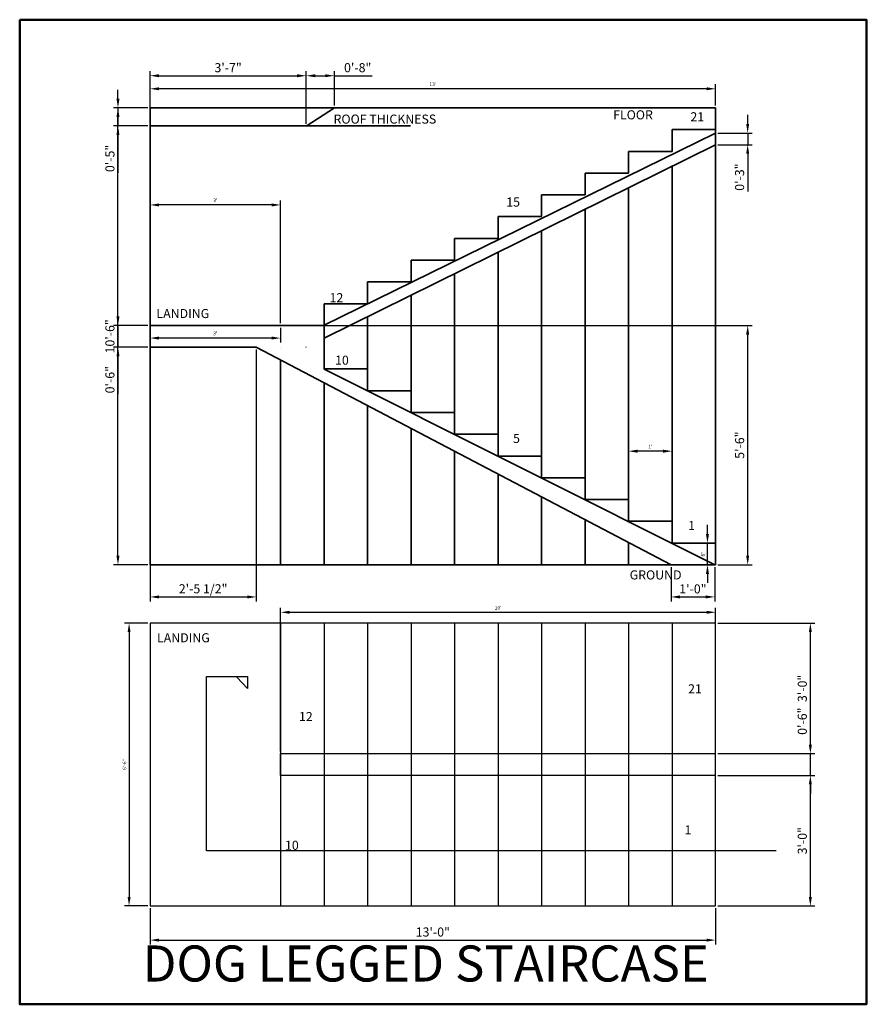
# Model space of a CAD drawing. Units: inches. Extents: x 183 to 417, y 53 to 324.
import ezdxf

# ---------------------------------------------------------------- set-up
doc = ezdxf.new("R2010")
doc.units = ezdxf.units.IN
for name, color, linetype, lineweight in [('A-ANNO-DIMS', 2, 'Continuous', 18), ('A-ANNO-TEXT', 7, 'Continuous', 25), ('A-ANNO-TTLB', 7, 'Continuous', 50), ('A-FLOR-STRS', 7, 'Continuous', 25), ('A-SECT', 7, 'Continuous', 35), ('A-SECT-PATT', 8, 'Continuous', 18)]:
    doc.layers.add(name, color=color, linetype=linetype, lineweight=lineweight)
doc.styles.get("Standard").update_dxf_attribs({"font": 'arial.ttf'})
doc.dimstyles.new('ISO-25', dxfattribs={"dimtxt": 2.5, "dimasz": 2.5, "dimexe": 1.25, "dimexo": 0.625, "dimtad": 1, "dimtxsty": 'Standard', "dimcen": 2.5, "dimadec": 0, "dimazin": 0, "dimtfac": 1, "dimtmove": 0, "dimatfit": 3, "dimfxl": 1, "dimarcsym": 0})

# ---------------------------------------------------------------- blocks, each defined once
blk = doc.blocks.new('*D1')
at = {"layer": 'A-ANNO-DIMS', "color": 0, "lineweight": -2, "transparency": 16777216}
for p, q in [((219.41, 300.49), (219.41, 306.37)), ((372.91, 305.12), (221.91, 305.12)), ((375.41, 300.49), (375.41, 306.37))]:
    blk.add_line(p, q, dxfattribs=at)
at = {"layer": 'A-ANNO-DIMS', "color": 0, "transparency": 16777216}
for points in [[(221.91, 305.54), (221.91, 304.7), (219.41, 305.12)], [(372.91, 305.54), (372.91, 304.7), (375.41, 305.12)]]:
    blk.add_solid(points, dxfattribs=at)
at = {"layer": 'Defpoints', "color": 0, "transparency": 16777216}
for p in [(219.41, 305.12), (219.41, 299.87), (375.41, 299.87)]:
    blk.add_point(p, dxfattribs=at)
at = {"layer": 'A-ANNO-DIMS', "color": 0, "transparency": 16777216, "insert": (297.41, 306.26), "char_height": 1, "attachment_point": 5}
blk.add_mtext("13'", dxfattribs=at)
blk = doc.blocks.new('*D2')
at = {"layer": 'A-ANNO-DIMS', "color": 0, "lineweight": -2, "transparency": 16777216}
for p, q in [((219.41, 240.49), (219.41, 274.35)), ((255.41, 240.49), (255.41, 274.35)), ((252.91, 273.1), (221.91, 273.1))]:
    blk.add_line(p, q, dxfattribs=at)
at = {"layer": 'A-ANNO-DIMS', "color": 0, "transparency": 16777216}
for points in [[(221.91, 273.51), (221.91, 272.68), (219.41, 273.1)], [(252.91, 273.51), (252.91, 272.68), (255.41, 273.1)]]:
    blk.add_solid(points, dxfattribs=at)
at = {"layer": 'Defpoints', "color": 0, "transparency": 16777216}
for p in [(219.41, 273.1), (219.41, 239.87), (255.41, 239.87)]:
    blk.add_point(p, dxfattribs=at)
at = {"layer": 'A-ANNO-DIMS', "color": 0, "transparency": 16777216, "insert": (237.41, 274.23), "char_height": 1, "attachment_point": 5}
blk.add_mtext("3'", dxfattribs=at)
blk = doc.blocks.new('*D3')
at = {"layer": 'A-ANNO-DIMS', "color": 0, "lineweight": -2, "transparency": 16777216}
for p, q in [((219.41, 239.24), (219.41, 235.14)), ((255.41, 239.24), (255.41, 235.14)), ((252.91, 236.39), (221.91, 236.39))]:
    blk.add_line(p, q, dxfattribs=at)
at = {"layer": 'A-ANNO-DIMS', "color": 0, "transparency": 16777216}
for points in [[(221.91, 236.81), (221.91, 235.97), (219.41, 236.39)], [(252.91, 236.81), (252.91, 235.97), (255.41, 236.39)]]:
    blk.add_solid(points, dxfattribs=at)
at = {"layer": 'Defpoints', "color": 0, "transparency": 16777216}
for p in [(219.41, 239.87), (255.41, 239.87), (219.41, 236.39)]:
    blk.add_point(p, dxfattribs=at)
at = {"layer": 'A-ANNO-DIMS', "color": 0, "transparency": 16777216, "insert": (237.41, 237.53), "char_height": 1, "attachment_point": 5}
blk.add_mtext("3'", dxfattribs=at)
blk = doc.blocks.new('*D4')
at = {"layer": 'A-ANNO-DIMS', "color": 0, "lineweight": -2, "transparency": 16777216}
for p, q in [((255.41, 122.44), (255.41, 162.04)), ((257.91, 160.79), (372.91, 160.79)), ((375.41, 122.44), (375.41, 162.04))]:
    blk.add_line(p, q, dxfattribs=at)
at = {"layer": 'A-ANNO-DIMS', "color": 0, "transparency": 16777216}
for points in [[(257.91, 161.2), (257.91, 160.37), (255.41, 160.79)], [(372.91, 161.2), (372.91, 160.37), (375.41, 160.79)]]:
    blk.add_solid(points, dxfattribs=at)
at = {"layer": 'Defpoints', "color": 0, "transparency": 16777216}
for p in [(375.41, 160.79), (255.41, 121.81), (375.41, 121.81)]:
    blk.add_point(p, dxfattribs=at)
at = {"layer": 'A-ANNO-DIMS', "color": 0, "transparency": 16777216, "insert": (315.41, 161.92), "char_height": 1, "attachment_point": 5}
blk.add_mtext("10'", dxfattribs=at)
blk = doc.blocks.new('*D5')
at = {"layer": 'A-ANNO-DIMS', "color": 0, "lineweight": -2, "transparency": 16777216}
for p, q in [((218.78, 157.81), (212.37, 157.81)), ((213.62, 155.31), (213.62, 82.31)), ((218.78, 79.81), (212.37, 79.81))]:
    blk.add_line(p, q, dxfattribs=at)
at = {"layer": 'A-ANNO-DIMS', "color": 0, "transparency": 16777216}
for points in [[(213.21, 155.31), (214.04, 155.31), (213.62, 157.81)], [(213.21, 82.31), (214.04, 82.31), (213.62, 79.81)]]:
    blk.add_solid(points, dxfattribs=at)
at = {"layer": 'Defpoints', "color": 0, "transparency": 16777216}
for p in [(219.41, 157.81), (213.62, 79.81), (219.41, 79.81)]:
    blk.add_point(p, dxfattribs=at)
at = {"layer": 'A-ANNO-DIMS', "color": 0, "transparency": 16777216, "insert": (212.49, 118.81), "char_height": 1, "attachment_point": 5, "rotation": 90}
blk.add_mtext('6\'-6"', dxfattribs=at)
blk = doc.blocks.new('*D6')
at = {"layer": 'A-ANNO-DIMS', "color": 0, "lineweight": -2, "transparency": 16777216}
for p, q in [((351.41, 186.49), (351.41, 206.45)), ((363.41, 186.49), (363.41, 206.45)), ((360.91, 205.2), (353.91, 205.2))]:
    blk.add_line(p, q, dxfattribs=at)
at = {"layer": 'A-ANNO-DIMS', "color": 0, "transparency": 16777216}
for points in [[(353.91, 205.62), (353.91, 204.78), (351.41, 205.2)], [(360.91, 205.62), (360.91, 204.78), (363.41, 205.2)]]:
    blk.add_solid(points, dxfattribs=at)
at = {"layer": 'Defpoints', "color": 0, "transparency": 16777216}
for p in [(351.41, 205.2), (351.41, 185.87), (363.41, 185.87)]:
    blk.add_point(p, dxfattribs=at)
at = {"layer": 'A-ANNO-DIMS', "color": 0, "transparency": 16777216, "insert": (357.41, 206.33), "char_height": 1, "attachment_point": 5}
blk.add_mtext("1'", dxfattribs=at)
blk = doc.blocks.new('*D7')
at = {"layer": 'A-ANNO-DIMS', "color": 0, "lineweight": -2, "transparency": 16777216}
for p, q in [((373.17, 182.37), (373.17, 184.87)), ((374.78, 179.87), (371.92, 179.87)), ((373.17, 173.87), (373.17, 179.87)), ((374.78, 173.87), (371.92, 173.87)), ((373.17, 171.37), (373.17, 168.87))]:
    blk.add_line(p, q, dxfattribs=at)
at = {"layer": 'A-ANNO-DIMS', "color": 0, "transparency": 16777216}
for points in [[(372.75, 182.37), (373.58, 182.37), (373.17, 179.87)], [(372.75, 171.37), (373.58, 171.37), (373.17, 173.87)]]:
    blk.add_solid(points, dxfattribs=at)
at = {"layer": 'Defpoints', "color": 0, "transparency": 16777216}
for p in [(373.17, 179.87), (375.41, 179.87), (375.41, 173.87)]:
    blk.add_point(p, dxfattribs=at)
at = {"layer": 'A-ANNO-DIMS', "color": 0, "transparency": 16777216, "insert": (372.03, 176.87), "char_height": 1, "attachment_point": 5, "rotation": 90}
blk.add_mtext('6"', dxfattribs=at)
blk = doc.blocks.new('*D8')
at = {"layer": 'A-ANNO-DIMS', "color": 0, "lineweight": -2, "transparency": 16777216}
for p, q in [((218.78, 299.87), (209.31, 299.87)), ((210.56, 176.37), (210.56, 297.37)), ((218.78, 173.87), (209.31, 173.87))]:
    blk.add_line(p, q, dxfattribs=at)
at = {"layer": 'A-ANNO-DIMS', "color": 0, "transparency": 16777216}
for points in [[(210.14, 297.37), (210.97, 297.37), (210.56, 299.87)], [(210.14, 176.37), (210.97, 176.37), (210.56, 173.87)]]:
    blk.add_solid(points, dxfattribs=at)
at = {"layer": 'Defpoints', "color": 0, "transparency": 16777216}
for p in [(210.56, 299.87), (219.41, 299.87), (219.41, 173.87)]:
    blk.add_point(p, dxfattribs=at)
at = {"layer": 'A-ANNO-DIMS', "color": 0, "transparency": 16777216, "insert": (208.66, 236.87), "char_height": 2.5, "attachment_point": 5, "rotation": 90}
blk.add_mtext('10\'-6"', dxfattribs=at)
blk = doc.blocks.new('*D9')
at = {"layer": 'A-ANNO-DIMS', "color": 0, "lineweight": -2, "transparency": 16777216}
for p, q in [((256.03, 239.87), (385.51, 239.87)), ((384.26, 176.37), (384.26, 237.37)), ((376.03, 173.87), (385.51, 173.87))]:
    blk.add_line(p, q, dxfattribs=at)
at = {"layer": 'A-ANNO-DIMS', "color": 0, "transparency": 16777216}
for points in [[(383.84, 237.37), (384.67, 237.37), (384.26, 239.87)], [(383.84, 176.37), (384.67, 176.37), (384.26, 173.87)]]:
    blk.add_solid(points, dxfattribs=at)
at = {"layer": 'Defpoints', "color": 0, "transparency": 16777216}
for p in [(255.41, 239.87), (384.26, 239.87), (375.41, 173.87)]:
    blk.add_point(p, dxfattribs=at)
at = {"layer": 'A-ANNO-DIMS', "color": 0, "transparency": 16777216, "insert": (382.36, 206.87), "char_height": 2.5, "attachment_point": 5, "rotation": 90}
blk.add_mtext('5\'-6"', dxfattribs=at)
blk = doc.blocks.new('*D10')
at = {"layer": 'A-ANNO-DIMS', "color": 0, "lineweight": -2, "transparency": 16777216}
for p, q in [((219.41, 79.19), (219.41, 69.16)), ((375.41, 79.19), (375.41, 69.16)), ((221.91, 70.41), (372.91, 70.41))]:
    blk.add_line(p, q, dxfattribs=at)
at = {"layer": 'A-ANNO-DIMS', "color": 0, "transparency": 16777216}
for points in [[(221.91, 70.83), (221.91, 69.99), (219.41, 70.41)], [(372.91, 70.83), (372.91, 69.99), (375.41, 70.41)]]:
    blk.add_solid(points, dxfattribs=at)
at = {"layer": 'Defpoints', "color": 0, "transparency": 16777216}
for p in [(219.41, 79.81), (375.41, 79.81), (375.41, 70.41)]:
    blk.add_point(p, dxfattribs=at)
at = {"layer": 'A-ANNO-DIMS', "color": 0, "transparency": 16777216, "insert": (297.41, 72.31), "char_height": 2.5, "attachment_point": 5}
blk.add_mtext('13\'-0"', dxfattribs=at)
blk = doc.blocks.new('*D11')
at = {"layer": 'A-ANNO-DIMS', "color": 0, "lineweight": -2, "transparency": 16777216}
for p, q in [((376.03, 115.81), (402.8, 115.81)), ((401.55, 82.31), (401.55, 113.31)), ((376.03, 79.81), (402.8, 79.81))]:
    blk.add_line(p, q, dxfattribs=at)
at = {"layer": 'A-ANNO-DIMS', "color": 0, "transparency": 16777216}
for points in [[(401.13, 113.31), (401.97, 113.31), (401.55, 115.81)], [(401.13, 82.31), (401.97, 82.31), (401.55, 79.81)]]:
    blk.add_solid(points, dxfattribs=at)
at = {"layer": 'Defpoints', "color": 0, "transparency": 16777216}
for p in [(375.41, 115.81), (401.55, 115.81), (375.41, 79.81)]:
    blk.add_point(p, dxfattribs=at)
at = {"layer": 'A-ANNO-DIMS', "color": 0, "transparency": 16777216, "insert": (399.65, 97.81), "char_height": 2.5, "attachment_point": 5, "rotation": 90}
blk.add_mtext('3\'-0"', dxfattribs=at)
blk = doc.blocks.new('*D12')
at = {"layer": 'A-ANNO-DIMS', "color": 0, "lineweight": -2, "transparency": 16777216}
for p, q in [((401.55, 124.31), (401.55, 134.71)), ((376.03, 121.81), (402.8, 121.81)), ((401.55, 115.81), (401.55, 121.81)), ((376.03, 115.81), (402.8, 115.81)), ((401.55, 113.31), (401.55, 110.81))]:
    blk.add_line(p, q, dxfattribs=at)
at = {"layer": 'A-ANNO-DIMS', "color": 0, "transparency": 16777216}
for points in [[(401.13, 124.31), (401.97, 124.31), (401.55, 121.81)], [(401.13, 113.31), (401.97, 113.31), (401.55, 115.81)]]:
    blk.add_solid(points, dxfattribs=at)
at = {"layer": 'Defpoints', "color": 0, "transparency": 16777216}
for p in [(375.41, 121.81), (401.55, 121.81), (375.41, 115.81)]:
    blk.add_point(p, dxfattribs=at)
at = {"layer": 'A-ANNO-DIMS', "color": 0, "transparency": 16777216, "insert": (399.65, 130.76), "char_height": 2.5, "attachment_point": 5, "rotation": 90}
blk.add_mtext('0\'-6"', dxfattribs=at)
blk = doc.blocks.new('*D13')
at = {"layer": 'A-ANNO-DIMS', "color": 0, "lineweight": -2, "transparency": 16777216}
for p, q in [((376.03, 157.81), (402.8, 157.81)), ((401.55, 124.31), (401.55, 155.31)), ((376.03, 121.81), (402.8, 121.81))]:
    blk.add_line(p, q, dxfattribs=at)
at = {"layer": 'A-ANNO-DIMS', "color": 0, "transparency": 16777216}
for points in [[(401.13, 155.31), (401.97, 155.31), (401.55, 157.81)], [(401.13, 124.31), (401.97, 124.31), (401.55, 121.81)]]:
    blk.add_solid(points, dxfattribs=at)
at = {"layer": 'Defpoints', "color": 0, "transparency": 16777216}
for p in [(375.41, 157.81), (401.55, 157.81), (375.41, 121.81)]:
    blk.add_point(p, dxfattribs=at)
at = {"layer": 'A-ANNO-DIMS', "color": 0, "transparency": 16777216, "insert": (399.65, 139.81), "char_height": 2.5, "attachment_point": 5, "rotation": 90}
blk.add_mtext('3\'-0"', dxfattribs=at)
blk = doc.blocks.new('*D14')
at = {"layer": 'A-ANNO-DIMS', "color": 0, "lineweight": -2, "transparency": 16777216}
for p, q in [((210.56, 302.37), (210.56, 304.87)), ((218.78, 299.87), (209.31, 299.87)), ((210.56, 299.87), (210.56, 294.87)), ((218.78, 294.87), (209.31, 294.87)), ((210.56, 292.37), (210.56, 281.97))]:
    blk.add_line(p, q, dxfattribs=at)
at = {"layer": 'A-ANNO-DIMS', "color": 0, "transparency": 16777216}
for points in [[(210.14, 302.37), (210.97, 302.37), (210.56, 299.87)], [(210.14, 292.37), (210.97, 292.37), (210.56, 294.87)]]:
    blk.add_solid(points, dxfattribs=at)
at = {"layer": 'Defpoints', "color": 0, "transparency": 16777216}
for p in [(219.41, 299.87), (210.56, 294.87), (219.41, 294.87)]:
    blk.add_point(p, dxfattribs=at)
at = {"layer": 'A-ANNO-DIMS', "color": 0, "transparency": 16777216, "insert": (208.66, 285.92), "char_height": 2.5, "attachment_point": 5, "rotation": 90}
blk.add_mtext('0\'-5"', dxfattribs=at)
blk = doc.blocks.new('*D15')
at = {"layer": 'A-ANNO-DIMS', "color": 0, "lineweight": -2, "transparency": 16777216}
for p, q in [((219.41, 295.49), (219.41, 309.97)), ((262.47, 295.49), (262.47, 309.97)), ((221.91, 308.72), (259.97, 308.72))]:
    blk.add_line(p, q, dxfattribs=at)
at = {"layer": 'A-ANNO-DIMS', "color": 0, "transparency": 16777216}
for points in [[(221.91, 309.14), (221.91, 308.3), (219.41, 308.72)], [(259.97, 309.14), (259.97, 308.3), (262.47, 308.72)]]:
    blk.add_solid(points, dxfattribs=at)
at = {"layer": 'Defpoints', "color": 0, "transparency": 16777216}
for p in [(262.47, 308.72), (219.41, 294.87), (262.47, 294.86)]:
    blk.add_point(p, dxfattribs=at)
at = {"layer": 'A-ANNO-DIMS', "color": 0, "transparency": 16777216, "insert": (240.94, 310.62), "char_height": 2.5, "attachment_point": 5}
blk.add_mtext('3\'-7"', dxfattribs=at)
blk = doc.blocks.new('*D16')
at = {"layer": 'A-ANNO-DIMS', "color": 0, "lineweight": -2, "transparency": 16777216}
for p, q in [((262.47, 295.49), (262.47, 309.97)), ((270.24, 300.49), (270.24, 309.97)), ((264.97, 308.72), (267.74, 308.72)), ((270.24, 308.72), (280.64, 308.72))]:
    blk.add_line(p, q, dxfattribs=at)
at = {"layer": 'A-ANNO-DIMS', "color": 0, "transparency": 16777216}
for points in [[(264.97, 309.14), (264.97, 308.3), (262.47, 308.72)], [(267.74, 309.14), (267.74, 308.3), (270.24, 308.72)]]:
    blk.add_solid(points, dxfattribs=at)
at = {"layer": 'Defpoints', "color": 0, "transparency": 16777216}
for p in [(270.24, 308.72), (270.24, 299.87), (262.47, 294.86)]:
    blk.add_point(p, dxfattribs=at)
at = {"layer": 'A-ANNO-DIMS', "color": 0, "transparency": 16777216, "insert": (276.69, 310.62), "char_height": 2.5, "attachment_point": 5}
blk.add_mtext('0\'-8"', dxfattribs=at)
blk = doc.blocks.new('*D17')
at = {"layer": 'A-ANNO-DIMS', "color": 0, "lineweight": -2, "transparency": 16777216}
for p, q in [((210.56, 242.37), (210.56, 244.87)), ((218.78, 239.87), (209.31, 239.87)), ((210.56, 239.87), (210.56, 233.87)), ((218.78, 233.87), (209.31, 233.87)), ((210.56, 231.37), (210.56, 220.97))]:
    blk.add_line(p, q, dxfattribs=at)
at = {"layer": 'A-ANNO-DIMS', "color": 0, "transparency": 16777216}
for points in [[(210.14, 242.37), (210.97, 242.37), (210.56, 239.87)], [(210.14, 231.37), (210.97, 231.37), (210.56, 233.87)]]:
    blk.add_solid(points, dxfattribs=at)
at = {"layer": 'Defpoints', "color": 0, "transparency": 16777216}
for p in [(219.41, 239.87), (210.56, 233.87), (219.41, 233.87)]:
    blk.add_point(p, dxfattribs=at)
at = {"layer": 'A-ANNO-DIMS', "color": 0, "transparency": 16777216, "insert": (208.66, 224.92), "char_height": 2.5, "attachment_point": 5, "rotation": 90}
blk.add_mtext('0\'-6"', dxfattribs=at)
blk = doc.blocks.new('*D18')
at = {"layer": 'A-ANNO-DIMS', "color": 0, "lineweight": -2, "transparency": 16777216}
for p, q in [((219.41, 233.24), (219.41, 163.77)), ((248.7, 233.24), (248.7, 163.77)), ((221.91, 165.02), (246.2, 165.02))]:
    blk.add_line(p, q, dxfattribs=at)
at = {"layer": 'A-ANNO-DIMS', "color": 0, "transparency": 16777216}
for points in [[(221.91, 165.44), (221.91, 164.6), (219.41, 165.02)], [(246.2, 165.44), (246.2, 164.6), (248.7, 165.02)]]:
    blk.add_solid(points, dxfattribs=at)
at = {"layer": 'Defpoints', "color": 0, "transparency": 16777216}
for p in [(219.41, 233.87), (248.7, 233.87), (248.7, 165.02)]:
    blk.add_point(p, dxfattribs=at)
at = {"layer": 'A-ANNO-DIMS', "color": 0, "transparency": 16777216, "insert": (234.05, 166.94), "char_height": 2.5, "attachment_point": 5}
blk.add_mtext('2\'-5 1/2"', dxfattribs=at)
blk = doc.blocks.new('*D19')
at = {"layer": 'A-ANNO-DIMS', "color": 0, "lineweight": -2, "transparency": 16777216}
for p, q in [((384.26, 295.42), (384.26, 297.92)), ((376.03, 292.92), (385.51, 292.92)), ((384.26, 292.92), (384.26, 289.71)), ((376.03, 289.71), (385.51, 289.71)), ((384.26, 287.21), (384.26, 276.81))]:
    blk.add_line(p, q, dxfattribs=at)
at = {"layer": 'A-ANNO-DIMS', "color": 0, "transparency": 16777216}
for points in [[(383.84, 295.42), (384.67, 295.42), (384.26, 292.92)], [(383.84, 287.21), (384.67, 287.21), (384.26, 289.71)]]:
    blk.add_solid(points, dxfattribs=at)
at = {"layer": 'Defpoints', "color": 0, "transparency": 16777216}
for p in [(375.41, 292.92), (375.41, 289.71), (384.26, 289.71)]:
    blk.add_point(p, dxfattribs=at)
at = {"layer": 'A-ANNO-DIMS', "color": 0, "transparency": 16777216, "insert": (382.35, 280.76), "char_height": 2.5, "attachment_point": 5, "rotation": 90}
blk.add_mtext('0\'-3"', dxfattribs=at)
blk = doc.blocks.new('*D20')
at = {"layer": 'A-ANNO-DIMS', "color": 0, "lineweight": -2, "transparency": 16777216}
for p, q in [((363.11, 173.24), (363.11, 163.77)), ((375.19, 173.24), (375.19, 163.77)), ((365.61, 165.02), (372.69, 165.02))]:
    blk.add_line(p, q, dxfattribs=at)
at = {"layer": 'A-ANNO-DIMS', "color": 0, "transparency": 16777216}
for points in [[(365.61, 165.44), (365.61, 164.6), (363.11, 165.02)], [(372.69, 165.44), (372.69, 164.6), (375.19, 165.02)]]:
    blk.add_solid(points, dxfattribs=at)
at = {"layer": 'Defpoints', "color": 0, "transparency": 16777216}
for p in [(363.11, 173.87), (375.19, 173.87), (375.19, 165.02)]:
    blk.add_point(p, dxfattribs=at)
at = {"layer": 'A-ANNO-DIMS', "color": 0, "transparency": 16777216, "insert": (369.15, 166.92), "char_height": 2.5, "attachment_point": 5}
blk.add_mtext('1\'-0"', dxfattribs=at)

msp = doc.modelspace()

# ---------------------------------------------------------------- hatches: boundary and pattern name
at = {"layer": 'A-SECT-PATT'}
h = msp.add_hatch(dxfattribs=at)
h.set_pattern_fill('AR-CONC', color=256, scale=0.9)
h.paths.add_polyline_path([(255.41, 239.87), (219.41, 239.87), (219.41, 233.87), (248.7, 233.87), (363.11, 173.87), (375.19, 173.87), (267.41, 227.85), (267.41, 233.87), (267.41, 239.87)])
h.paths.add_polyline_path([(255.41, 233.87), (255.41, 233.86), (255.4, 233.87)], flags=16)
h = msp.add_hatch(dxfattribs=at)
h.set_pattern_fill('AR-CONC', color=256, scale=0.9)
h.paths.add_polyline_path([(255.41, 239.87), (219.41, 239.87), (219.41, 233.87), (248.7, 233.87), (363.11, 173.87), (375.19, 173.87), (267.37, 227.87), (267.41, 227.87), (267.41, 233.87), (267.41, 239.87)])
h.paths.add_polyline_path([(255.4, 233.87), (255.41, 233.87), (255.41, 233.86)], flags=16)

# ---------------------------------------------------------------- linework, layer by layer
at = {"layer": 'A-ANNO-TTLB'}
msp.add_lwpolyline([(183.44, 324.17), (416.99, 324.17), (416.99, 52.71), (183.44, 52.71)], close=True, dxfattribs=at)
at = {"layer": 'A-FLOR-STRS'}
for p, q in [((375.41, 157.81), (219.41, 157.81)), ((219.41, 157.81), (219.41, 79.81)), ((255.41, 157.81), (255.41, 79.81)), ((267.41, 157.81), (267.41, 79.81)), ((279.41, 157.81), (279.41, 79.81)), ((291.41, 157.81), (291.41, 79.81)), ((303.41, 157.81), (303.41, 79.81)), ((315.41, 157.81), (315.41, 79.81)), ((327.41, 157.81), (327.41, 79.81)), ((339.41, 157.81), (339.41, 79.81)), ((351.41, 157.81), (351.41, 79.81)), ((363.41, 157.81), (363.41, 79.81)), ((375.41, 115.81), (375.41, 157.81)), ((234.95, 95.04), (234.95, 143.12)), ((234.95, 143.12), (246.33, 143.12)), ((246.33, 139.78), (243.39, 142.89)), ((246.33, 143.12), (246.33, 139.78)), ((255.41, 115.81), (255.41, 121.81)), ((255.41, 121.81), (375.41, 121.81)), ((375.41, 79.81), (375.41, 121.81)), ((375.41, 115.81), (255.41, 115.81)), ((392.15, 95.04), (234.95, 95.04)), ((219.41, 79.81), (375.41, 79.81))]:
    msp.add_line(p, q, dxfattribs=at)
at = {"layer": 'A-SECT'}
for p, q in [((219.41, 299.87), (219.41, 173.87)), ((375.41, 299.87), (219.41, 299.87)), ((262.47, 294.86), (270.24, 299.87)), ((375.41, 173.87), (375.41, 299.87)), ((375.41, 293.87), (375.41, 299.87)), ((291.26, 294.87), (219.41, 294.87)), ((363.41, 287.87), (363.41, 293.87)), ((363.41, 293.87), (375.41, 293.87)), ((267.28, 239.87), (375.41, 292.92)), ((267.41, 236.32), (375.41, 289.71)), ((351.41, 281.87), (351.41, 287.87)), ((351.41, 287.87), (363.41, 287.87)), ((363.41, 179.77), (363.41, 283.77)), ((339.41, 275.87), (339.41, 281.87)), ((339.41, 281.87), (351.41, 281.87)), ((351.41, 277.84), (351.41, 185.78)), ((327.41, 269.87), (327.41, 275.87)), ((327.41, 275.87), (339.41, 275.87)), ((339.41, 271.91), (339.41, 191.79)), ((315.41, 263.87), (315.41, 269.87)), ((315.41, 269.87), (327.41, 269.87)), ((303.41, 257.87), (303.41, 263.87)), ((303.41, 263.87), (315.41, 263.87)), ((327.41, 265.98), (327.41, 197.8)), ((315.41, 260.05), (315.41, 203.81)), ((291.41, 251.87), (291.41, 257.87)), ((291.41, 257.87), (303.41, 257.87)), ((291.41, 257.87), (291.41, 251.7)), ((303.41, 254.12), (303.41, 209.82)), ((279.41, 245.87), (279.41, 251.87)), ((279.41, 251.87), (291.41, 251.87)), ((291.41, 248.18), (291.41, 215.83)), ((267.41, 239.87), (267.41, 245.87)), ((267.41, 245.87), (279.41, 245.87)), ((279.41, 242.25), (279.41, 221.84)), ((255.41, 239.87), (219.41, 239.87)), ((255.41, 239.87), (267.41, 239.87)), ((267.41, 239.93), (267.41, 227.85)), ((248.7, 233.87), (219.41, 233.87)), ((248.7, 233.87), (363.11, 173.87)), ((255.41, 233.87), (255.4, 233.87)), ((255.4, 233.87), (255.41, 233.86)), ((255.41, 233.87), (255.41, 233.86)), ((255.41, 233.87), (255.41, 233.86)), ((262.4, 233.84), (262.45, 233.87)), ((267.41, 227.87), (267.41, 233.87)), ((255.41, 230.35), (255.41, 173.87)), ((279.41, 227.87), (267.41, 227.87)), ((267.41, 227.87), (267.41, 227.85)), ((267.41, 227.85), (375.19, 173.87)), ((279.41, 221.87), (279.41, 227.87)), ((267.41, 224.06), (267.41, 173.87)), ((291.41, 221.87), (279.41, 221.87)), ((279.41, 221.87), (279.41, 221.84)), ((291.41, 215.87), (291.41, 221.87)), ((279.41, 217.77), (279.41, 173.87)), ((303.41, 215.87), (291.41, 215.87)), ((291.41, 215.87), (291.41, 215.83)), ((303.41, 209.87), (303.41, 215.87)), ((291.41, 211.47), (291.41, 173.87)), ((315.41, 209.87), (303.41, 209.87)), ((303.41, 209.87), (303.41, 209.82)), ((315.41, 203.87), (315.41, 209.87)), ((303.41, 205.18), (303.41, 173.87)), ((327.41, 203.87), (315.41, 203.87)), ((315.41, 203.87), (315.41, 203.81)), ((327.41, 197.87), (327.41, 203.87)), ((315.41, 198.88), (315.41, 173.87)), ((339.41, 197.87), (327.41, 197.87)), ((327.41, 197.87), (327.41, 197.8)), ((339.41, 191.87), (339.41, 197.87)), ((327.41, 192.59), (327.41, 173.87)), ((351.41, 191.87), (339.41, 191.87)), ((339.41, 191.87), (339.41, 191.79)), ((351.41, 185.87), (351.41, 191.87)), ((339.41, 186.3), (339.41, 173.87)), ((363.41, 185.87), (351.41, 185.87)), ((351.41, 185.87), (351.41, 185.78)), ((351.41, 180), (351.41, 173.87)), ((375.41, 179.87), (363.41, 179.87)), ((363.41, 179.87), (363.41, 179.77)), ((375.41, 173.87), (375.41, 179.87)), ((375.41, 173.87), (219.41, 173.87))]:
    msp.add_line(p, q, dxfattribs=at)

# ---------------------------------------------------------------- texts
at = {"layer": 'A-ANNO-TEXT', "attachment_point": 1}
for s, width, gutter_width, insert, char_height in [('FLOOR', 11.2408, 12.5, (347.14, 299.19), 2.5), ('21', 4.2515, 12.5, (368.46, 298.65), 2.5), ('ROOF THICKNESS', 33.3055, 12.5, (270.03, 298.01), 2.5), ('15', 6.125, 12.5, (317.67, 275.15), 2.5), ('12 ', 6.0758, 12.5, (268.93, 248.78), 2.5), ('LANDING', 38.6573, 12.5, (221.17, 244.41), 2.5), ('10', 5.9922, 12.5, (270.44, 231.55), 2.5), ('5', 5.0121, 12.5, (319.54, 209.97), 2.5), ('1', 4.5271, 12.5, (367.82, 185.95), 2.5), ('GROUND', 27.4098, 12.5, (351.71, 172.34), 2.5), ('LANDING', 32.9045, 12.5, (221.33, 155.01), 2.5), ('21', 3.431, 12.5, (367.83, 140.94), 2.5), ('12', 3.1135, 12.5, (260.48, 133.3), 2.5), ('1', 4.8197, 12.5, (366.85, 102.05), 2.5), ('10', 4.6702, 12.5, (256.63, 97.8), 2.5), ('DOG LEGGED STAIRCASE', 665.7442, 49.71, (217.36, 68.93), 9.9414)]:
    msp.add_mtext_dynamic_manual_height_columns(s, width=width, gutter_width=gutter_width, heights=[0], dxfattribs=dict(at, insert=insert, char_height=char_height))

# ---------------------------------------------------------------- dimensions: what is measured, and where the dimension line sits
at = {"layer": 'A-ANNO-DIMS'}
for base, p1, p2, override, picture, middle in [((262.47, 308.72), (219.41, 294.87), (262.47, 294.86), {"dimdec": 1, "dimlfac": 1, "dimrnd": 0, "dimzin": 1, "dimdsep": 46, "dimlunit": 4, "dimfrac": 2}, '*D15', (240.94, 310.62)), ((270.24, 308.72), (262.47, 294.86), (270.24, 299.87), {"dimdec": 1, "dimlfac": 1, "dimrnd": 0, "dimzin": 1, "dimdsep": 46, "dimlunit": 4, "dimfrac": 2}, '*D16', (276.69, 310.62)), ((219.41, 305.12), (375.41, 299.87), (219.41, 299.87), {"dimtxt": 1, "dimdec": 0, "dimlunit": 3, "dimclrd": 0, "dimclre": 0, "dimclrt": 0, "dimtdec": 0}, '*D1', (297.41, 306.26)), ((219.41, 273.1), (255.41, 239.87), (219.41, 239.87), {"dimtxt": 1, "dimdec": 0, "dimlunit": 3, "dimclrd": 0, "dimclre": 0, "dimclrt": 0, "dimtdec": 0}, '*D2', (237.41, 274.23)), ((219.41, 236.39), (255.41, 239.87), (219.41, 239.87), {"dimtxt": 1, "dimdec": 0, "dimlunit": 3, "dimclrd": 0, "dimclre": 0, "dimclrt": 0, "dimtdec": 0}, '*D3', (237.41, 237.53)), ((248.7, 165.02), (219.41, 233.87), (248.7, 233.87), {"dimdec": 1, "dimlfac": 1, "dimrnd": 0, "dimzin": 1, "dimdsep": 46, "dimlunit": 4, "dimfrac": 2}, '*D18', (234.05, 166.94)), ((351.41, 205.2), (363.41, 185.87), (351.41, 185.87), {"dimtxt": 1, "dimdec": 0, "dimlunit": 3, "dimclrd": 0, "dimclre": 0, "dimclrt": 0, "dimtdec": 0}, '*D6', (357.41, 206.33)), ((375.19, 165.02), (363.11, 173.87), (375.19, 173.87), {"dimdec": 1, "dimlfac": 1, "dimrnd": 0, "dimzin": 1, "dimdsep": 46, "dimlunit": 4, "dimfrac": 2}, '*D20', (369.15, 166.92)), ((375.41, 160.79), (255.41, 121.81), (375.41, 121.81), {"dimtxt": 1, "dimdec": 0, "dimlunit": 3, "dimclrd": 0, "dimclre": 0, "dimclrt": 0, "dimtdec": 0}, '*D4', (315.41, 161.92)), ((375.41, 70.41), (219.41, 79.81), (375.41, 79.81), {"dimdec": 1, "dimlfac": 1, "dimrnd": 0, "dimzin": 1, "dimdsep": 46, "dimlunit": 4, "dimfrac": 2}, '*D10', (297.41, 72.31))]:
    dim = msp.add_linear_dim(base=base, p1=p1, p2=p2, dimstyle='ISO-25', override=override, dxfattribs=at)
    dim.commit()
    dim.dimension.update_dxf_attribs({"geometry": picture, "text_midpoint": middle})
for base, p1, p2, override, picture, middle in [((210.56, 294.87), (219.41, 299.87), (219.41, 294.87), {"dimdec": 1, "dimlfac": 1, "dimrnd": 0, "dimzin": 1, "dimdsep": 46, "dimlunit": 4, "dimfrac": 2}, '*D14', (208.66, 285.92)), ((210.56, 299.87), (219.41, 173.87), (219.41, 299.87), {"dimdec": 1, "dimlfac": 1, "dimrnd": 0, "dimzin": 1, "dimdsep": 46, "dimlunit": 4, "dimfrac": 2}, '*D8', (208.66, 236.87)), ((384.26, 289.71), (375.41, 292.92), (375.41, 289.71), {"dimdec": 1, "dimlfac": 1, "dimrnd": 0, "dimzin": 1, "dimdsep": 46, "dimlunit": 4, "dimfrac": 2}, '*D19', (382.35, 280.76)), ((210.56, 233.87), (219.41, 239.87), (219.41, 233.87), {"dimdec": 1, "dimlfac": 1, "dimrnd": 0, "dimzin": 1, "dimdsep": 46, "dimlunit": 4, "dimfrac": 2}, '*D17', (208.66, 224.92)), ((384.26, 239.87), (375.41, 173.87), (255.41, 239.87), {"dimdec": 1, "dimlfac": 1, "dimrnd": 0, "dimzin": 1, "dimdsep": 46, "dimlunit": 4, "dimfrac": 2}, '*D9', (382.36, 206.87)), ((373.17, 179.87), (375.41, 173.87), (375.41, 179.87), {"dimtxt": 1, "dimdec": 0, "dimlunit": 3, "dimclrd": 0, "dimclre": 0, "dimclrt": 0, "dimtdec": 0}, '*D7', (372.03, 176.87)), ((213.62, 79.81), (219.41, 157.81), (219.41, 79.81), {"dimtxt": 1, "dimdec": 0, "dimlunit": 3, "dimclrd": 0, "dimclre": 0, "dimclrt": 0, "dimtdec": 0}, '*D5', (212.49, 118.81)), ((401.55, 157.81), (375.41, 121.81), (375.41, 157.81), {"dimdec": 1, "dimlfac": 1, "dimrnd": 0, "dimzin": 1, "dimdsep": 46, "dimlunit": 4, "dimfrac": 2}, '*D13', (399.65, 139.81)), ((401.55, 121.81), (375.41, 115.81), (375.41, 121.81), {"dimdec": 1, "dimlfac": 1, "dimrnd": 0, "dimzin": 1, "dimdsep": 46, "dimlunit": 4, "dimfrac": 2}, '*D12', (399.65, 130.76)), ((401.55, 115.81), (375.41, 79.81), (375.41, 115.81), {"dimdec": 1, "dimlfac": 1, "dimrnd": 0, "dimzin": 1, "dimdsep": 46, "dimlunit": 4, "dimfrac": 2}, '*D11', (399.65, 97.81))]:
    dim = msp.add_linear_dim(base=base, p1=p1, p2=p2, angle=90, dimstyle='ISO-25', override=override, dxfattribs=at)
    dim.commit()
    dim.dimension.update_dxf_attribs({"geometry": picture, "text_midpoint": middle})

doc.saveas('drawing.dxf')
